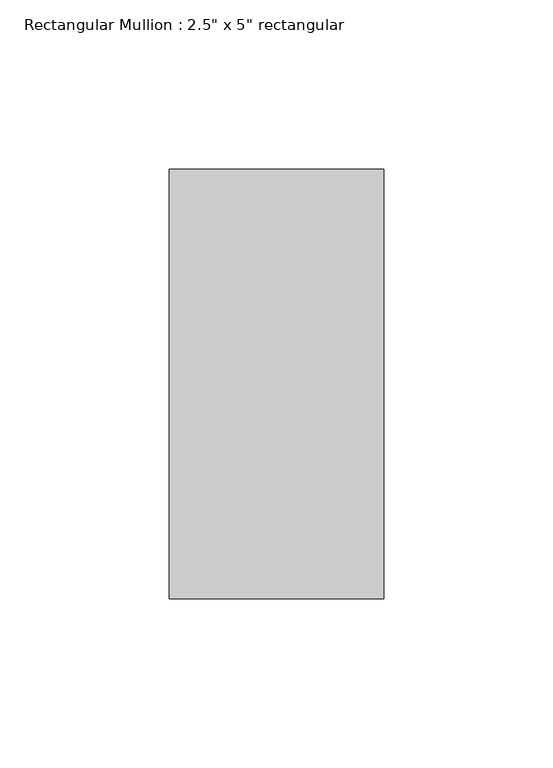
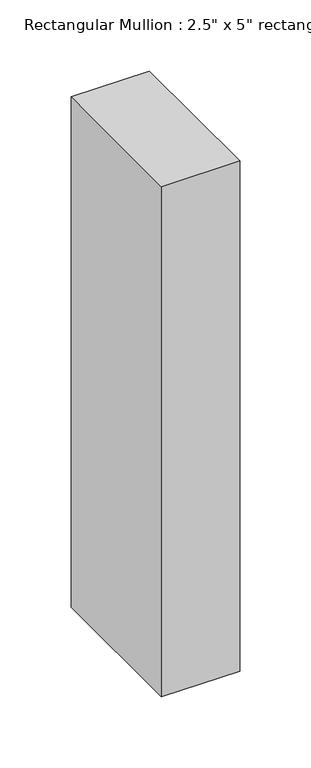
"""IFC4 building model written with IfcOpenShell, lengths in millimetres: member geometry."""

from ifc_helpers import new_model, si_unit, frame, origin, place, context, project, spatial, polyline, outline, extrude, source, transform, mapped, element, save


def member_6fb4a552(model_context):
    return source(origin(), model_context, "Body", "SweptSolid", [
        extrude(outline(polyline([(0.0, 63.5), (0.0, -63.5), (-63.5, -63.5), (-63.5, 63.5), (0.0, 63.5)])), frame((0.0, 0.0, -438.15), z_axis=(0.0, 0.0, 1.0), x_axis=(1.0, 0.0, 0.0)), (0.0, 0.0, 1.0), 438.15),
    ])


if __name__ == "__main__":
    model = new_model("IFC4")
    model_context = context("Model", 3, world=origin())
    ifc_project = project(units=[si_unit("LENGTHUNIT", "METRE", prefix="MILLI")], contexts=[model_context])
    site = spatial("IfcSite", under=ifc_project)
    building = spatial("IfcBuilding", under=site)
    placement = place(None, origin())
    member_shape = member_6fb4a552(model_context)
    element("IfcMember", 1, ObjectType="Rectangular Mullion : 2.5\" x 5\" rectangular", at=placement, inside=building, context=model_context, shape_type="MappedRepresentation", body=[
        mapped(member_shape, transform((0.0, 0.0, 0.0), x_axis=(1.0, 0.0, 0.0), y_axis=(0.0, 1.0, 0.0), z_axis=(0.0, 0.0, 1.0))),
    ])
    save(model, "model.ifc")

# Revit data of these elements
# Type "Rectangular Mullion : 2.5\" x 5\" rectangular"
#   built-in parameter 1007304 = 0.416667 (stored number, unit not read)
#   built-in parameter 1007301 = 0.104167 (stored number, unit not read)
#   built-in parameter 1007300 = 0.104167 (stored number, unit not read)
# Element 1 (IfcMember, "Rectangular Mullion : 2.5\" x 5\" rectangular")
#   Materials on its faces: "Aluminum"
# Materials
#   "Aluminum": class "Metal", colour RGB 247 247 247, transparency 0, Description = "Aluminum 6061", Cost = 0
